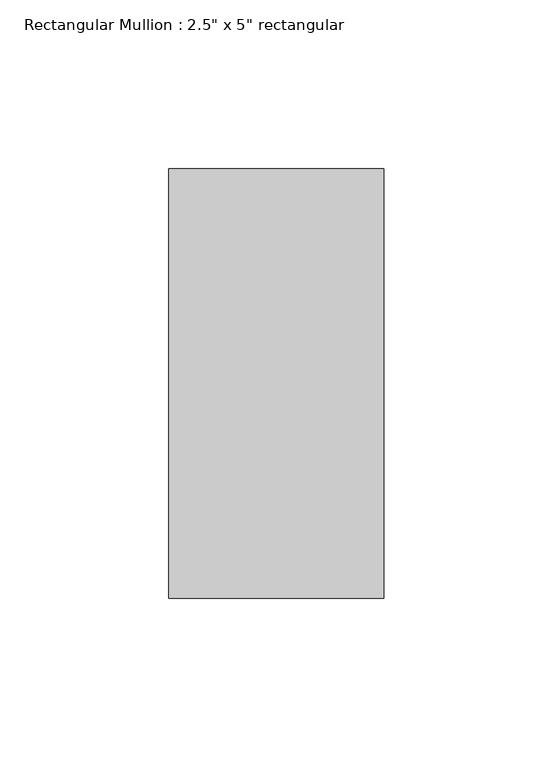
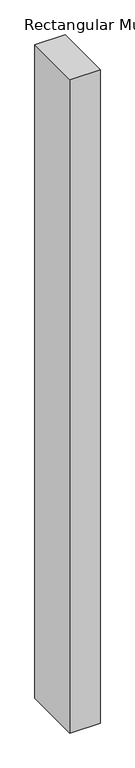
"""IFC4 building model written with IfcOpenShell, lengths in millimetres: member geometry."""

from ifc_helpers import new_model, si_unit, frame, origin, place, context, project, spatial, polyline, outline, extrude, source, transform, mapped, element, save


def member_c59792e9(model_context):
    return source(origin(), model_context, "Body", "SweptSolid", [
        extrude(outline(polyline([(0.0, 63.5), (0.0, -63.5), (-63.5, -63.5), (-63.5, 63.5), (0.0, 63.5)])), frame((0.0, 0.0, -1451.8907014), z_axis=(0.0, 0.0, 1.0), x_axis=(1.0, 0.0, 0.0)), (0.0, 0.0, 1.0), 1451.8907014),
    ])


if __name__ == "__main__":
    model = new_model("IFC4")
    model_context = context("Model", 3, world=origin())
    ifc_project = project(units=[si_unit("LENGTHUNIT", "METRE", prefix="MILLI")], contexts=[model_context])
    site = spatial("IfcSite", under=ifc_project)
    building = spatial("IfcBuilding", under=site)
    placement = place(None, origin())
    member_shape = member_c59792e9(model_context)
    element("IfcMember", 1, ObjectType="Rectangular Mullion : 2.5\" x 5\" rectangular", at=placement, inside=building, context=model_context, shape_type="MappedRepresentation", body=[
        mapped(member_shape, transform((0.0, 0.0, 0.0), x_axis=(1.0, 0.0, 0.0), y_axis=(0.0, 1.0, 0.0), z_axis=(0.0, 0.0, 1.0))),
    ])
    save(model, "model.ifc")

# Revit data of these elements
# Type "Rectangular Mullion : 2.5\" x 5\" rectangular"
#   built-in parameter 1007304 = 0.416667 (stored number, unit not read)
#   built-in parameter 1007301 = 0.104167 (stored number, unit not read)
#   built-in parameter 1007300 = 0.104167 (stored number, unit not read)
# Element 1 (IfcMember, "Rectangular Mullion : 2.5\" x 5\" rectangular")
#   Materials on its faces: "Aluminum"
# Materials
#   "Aluminum": class "Metal", colour RGB 247 247 247, transparency 0, Description = "Aluminum 6061", Cost = 0
